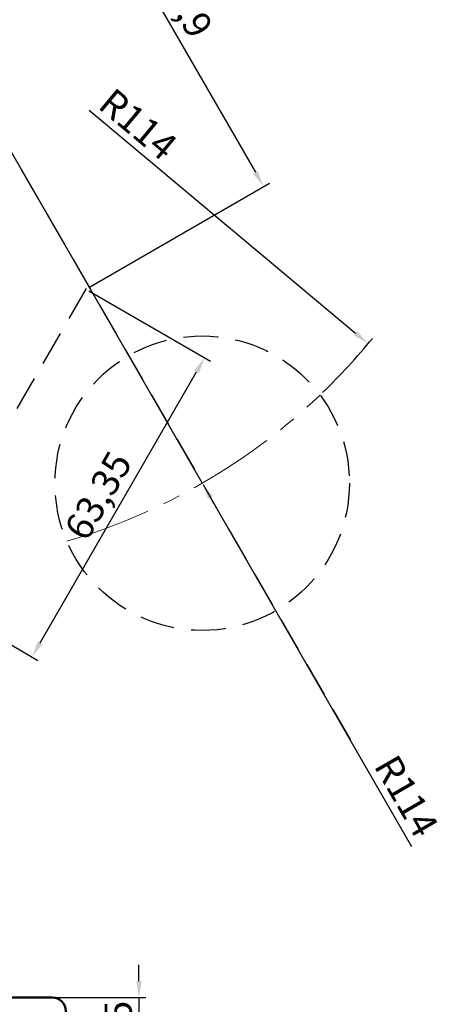
# Model space of a CAD drawing. Units: millimetres. Extents: x 98 to 674, y 38 to 476.
# Tile 5 of 7: x 315 to 392, y 131 to 312. Entities that reach past the tile are written whole.
import ezdxf

# ---------------------------------------------------------------- set-up
doc = ezdxf.new("R2010")
doc.units = ezdxf.units.MM
doc.header["$LTSCALE"] = 0.5
doc.linetypes.add('CENTER', pattern=[50.8, 31.75, -6.35, 6.35, -6.35])
doc.linetypes.add('DASHED', pattern=[19.05, 12.7, -6.35])
for name, color, linetype, lineweight in [('M-CNTR', 1, 'CENTER', 18), ('M-DIMS', 2, 'Continuous', 25), ('M-OUTL', 7, 'Continuous', 50), ('M-PHAN', 6, 'DASHED', 25)]:
    doc.layers.add(name, color=color, linetype=linetype, lineweight=lineweight)
doc.styles.get("Standard").update_dxf_attribs({"font": 'arial.ttf'})
doc.dimstyles.new('ISO-25', dxfattribs={"dimtxt": 5, "dimasz": 3, "dimexe": 1.25, "dimexo": 0.625, "dimtad": 1, "dimtxsty": 'Standard', "dimcen": 2.5, "dimadec": 0, "dimazin": 0, "dimtfac": 1, "dimtmove": 0, "dimatfit": 3, "dimfxl": 1, "dimarcsym": 0})

# ---------------------------------------------------------------- blocks, each defined once
blk = doc.blocks.new('*D20')
at = {"layer": 'Defpoints', "color": 0, "ltscale": 0.5, "transparency": 16777216}
for p in [(290.59, 325.69), (359.62, 281.36), (327.04, 262.55)]:
    blk.add_point(p, dxfattribs=at)
at = {"layer": 'M-DIMS', "color": 0, "lineweight": -2, "ltscale": 0.5, "transparency": 16777216}
for p, q in [((291.13, 326), (324.25, 345.12)), ((324.67, 341.9), (358.12, 283.96)), ((327.58, 262.86), (360.7, 281.99))]:
    blk.add_line(p, q, dxfattribs=at)
at = {"layer": 'M-DIMS', "color": 0, "ltscale": 0.5, "transparency": 16777216}
for points in [[(325.1, 342.15), (324.24, 341.65), (323.17, 344.5)], [(358.56, 284.21), (357.69, 283.71), (359.62, 281.36)]]:
    blk.add_solid(points, dxfattribs=at)
at = {"layer": 'M-DIMS', "color": 0, "ltscale": 0.5, "transparency": 16777216, "insert": (344.54, 314.74), "char_height": 5, "attachment_point": 5, "rotation": 300}
blk.add_mtext('72,9', dxfattribs=at)
blk = doc.blocks.new('*D21')
at = {"layer": 'Defpoints', "color": 0, "ltscale": 0.5, "transparency": 16777216}
for p in [(327.04, 262.55), (348.82, 249.98), (295.37, 207.69)]:
    blk.add_point(p, dxfattribs=at)
at = {"layer": 'M-DIMS', "color": 0, "lineweight": -2, "ltscale": 0.5, "transparency": 16777216}
for p, q in [((327.58, 262.24), (349.9, 249.35)), ((318.64, 197.71), (347.32, 247.38)), ((295.91, 207.37), (318.22, 194.49))]:
    blk.add_line(p, q, dxfattribs=at)
at = {"layer": 'M-DIMS', "color": 0, "ltscale": 0.5, "transparency": 16777216}
for points in [[(346.89, 247.63), (347.75, 247.13), (348.82, 249.98)], [(318.21, 197.96), (319.08, 197.46), (317.14, 195.11)]]:
    blk.add_solid(points, dxfattribs=at)
at = {"layer": 'M-DIMS', "color": 0, "ltscale": 0.5, "transparency": 16777216, "insert": (329.84, 224.36), "char_height": 5, "attachment_point": 5, "rotation": 60}
blk.add_mtext('63,35', dxfattribs=at)
blk = doc.blocks.new('*D22')
at = {"layer": 'Defpoints', "color": 0, "ltscale": 0.5, "transparency": 16777216}
for p in [(291.37, 325.69), (378.81, 252.55)]:
    blk.add_point(p, dxfattribs=at)
at = {"layer": 'M-DIMS', "color": 0, "lineweight": -2, "ltscale": 0.5, "transparency": 16777216}
blk.add_line((327.65, 295.34), (376.51, 254.47), dxfattribs=at)
blk.add_arc((291.37, 325.69), 114, 313.9161, 320.7202, dxfattribs=at)
at = {"layer": 'M-DIMS', "color": 0, "ltscale": 0.5, "transparency": 16777216}
blk.add_solid([(376.83, 254.86), (376.19, 254.09), (378.81, 252.55)], dxfattribs=at)
at = {"layer": 'M-DIMS', "color": 0, "ltscale": 0.5, "transparency": 16777216, "insert": (336.2, 292.27), "char_height": 5, "attachment_point": 5, "rotation": 320.0919}
blk.add_mtext('R114', dxfattribs=at)
blk = doc.blocks.new('*D42')
at = {"layer": 'Defpoints', "color": 0, "ltscale": 0.5, "transparency": 16777216}
for p in [(316.66, 132.69), (316.66, 127.69), (336.77, 127.69)]:
    blk.add_point(p, dxfattribs=at)
at = {"layer": 'M-DIMS', "color": 0, "lineweight": -2, "ltscale": 0.5, "transparency": 16777216}
for p, q in [((336.77, 135.69), (336.77, 138.69)), ((317.29, 132.69), (338.02, 132.69)), ((336.77, 132.69), (336.77, 127.69)), ((317.29, 127.69), (338.02, 127.69)), ((336.77, 124.69), (336.77, 121.69))]:
    blk.add_line(p, q, dxfattribs=at)
at = {"layer": 'M-DIMS', "color": 0, "ltscale": 0.5, "transparency": 16777216}
for points in [[(336.27, 135.69), (337.27, 135.69), (336.77, 132.69)], [(336.27, 124.69), (337.27, 124.69), (336.77, 127.69)]]:
    blk.add_solid(points, dxfattribs=at)
at = {"layer": 'M-DIMS', "color": 0, "ltscale": 0.5, "transparency": 16777216, "insert": (333.6, 130.19), "char_height": 5, "attachment_point": 5, "rotation": 90}
blk.add_mtext('5', dxfattribs=at)
blk = doc.blocks.new('*D72')
at = {"layer": 'Defpoints', "color": 0, "ltscale": 0.5, "transparency": 16777216}
for p in [(149.37, 196.69), (323.37, 130.19), (323.37, 42.76)]:
    blk.add_point(p, dxfattribs=at)
at = {"layer": 'M-DIMS', "color": 0, "lineweight": -2, "ltscale": 0.5, "transparency": 16777216}
for p, q in [((149.37, 196.06), (149.37, 41.51)), ((323.37, 129.56), (323.37, 41.51)), ((152.37, 42.76), (320.37, 42.76))]:
    blk.add_line(p, q, dxfattribs=at)
at = {"layer": 'M-DIMS', "color": 0, "ltscale": 0.5, "transparency": 16777216}
for points in [[(152.37, 43.26), (152.37, 42.26), (149.37, 42.76)], [(320.37, 43.26), (320.37, 42.26), (323.37, 42.76)]]:
    blk.add_solid(points, dxfattribs=at)
at = {"layer": 'M-DIMS', "color": 0, "ltscale": 0.5, "transparency": 16777216, "insert": (236.37, 45.9), "char_height": 5, "attachment_point": 5}
blk.add_mtext('174', dxfattribs=at)
blk = doc.blocks.new('*D78')
at = {"layer": 'Defpoints', "color": 0, "ltscale": 0.5, "transparency": 16777216}
for p in [(291.37, 325.69), (348.37, 226.96)]:
    blk.add_point(p, dxfattribs=at)
at = {"layer": 'M-DIMS', "color": 0, "lineweight": -2, "ltscale": 0.5, "transparency": 16777216}
for p, q in [((291.37, 325.69), (348.37, 226.96)), ((386.83, 160.33), (349.87, 224.36))]:
    blk.add_line(p, q, dxfattribs=at)
at = {"layer": 'M-DIMS', "color": 0, "ltscale": 0.5, "transparency": 16777216}
blk.add_solid([(350.3, 224.61), (349.43, 224.11), (348.37, 226.96)], dxfattribs=at)
at = {"layer": 'M-DIMS', "color": 0, "ltscale": 0.5, "transparency": 16777216, "insert": (385.28, 169.29), "char_height": 5, "attachment_point": 5, "rotation": 300.0001}
blk.add_mtext('R114', dxfattribs=at)

msp = doc.modelspace()

# ---------------------------------------------------------------- linework, layer by layer
at = {"layer": 'M-CNTR'}
msp.add_arc((291.365, 325.6855), 114, 286.398028, 313.601972, dxfattribs=at)
at = {"layer": 'M-OUTL'}
msp.add_lwpolyline([(320.865, 132.6855), (233.865, 132.6855, 1), (233.865, 127.6855), (320.865, 127.6855, 1)], format="xyb", close=True, dxfattribs=at)
at = {"layer": 'M-PHAN'}
for p, q in [((291.365, 325.6855), (375.7053, 179.6039)), ((295.365, 207.6855), (327.4287, 263.2214))]:
    msp.add_line(p, q, dxfattribs=at)
msp.add_circle((348.365, 226.9586), 27, dxfattribs=at)

# ---------------------------------------------------------------- dimensions: what is measured, and where the dimension line sits
at = {"layer": 'M-DIMS', "ltscale": 0.5}
for p1, distance, picture, middle in [((290.5915, 325.6855), 37.6203, '*D20', (344.5403, 314.7435)), ((295.365, 207.6855), -25.146, '*D21', (329.8371, 224.3604))]:
    dim = msp.add_aligned_dim(p1=p1, p2=(327.0419, 262.5515), distance=distance, dimstyle='ISO-25', override={"dimclrd": 0, "dimclre": 0, "dimclrt": 0}, dxfattribs=at)
    dim.commit()
    dim.dimension.update_dxf_attribs({"geometry": picture, "text_midpoint": middle})
for mpoint, override, picture, middle in [((378.8115, 252.5479), {"dimclrd": 0, "dimclre": 0, "dimclrt": 0}, '*D22', (334.1894, 289.8685)), ((348.3652, 226.9587), {"dimdec": 0, "dimlfac": 1, "dimrnd": 0, "dimzin": 0, "dimdsep": 46, "dimlunit": 2}, '*D78', (382.5653, 167.7226))]:
    dim = msp.add_radius_dim(center=(291.365, 325.6855), mpoint=mpoint, dimstyle='ISO-25', override=override, dxfattribs=at)
    dim.commit()
    dim.dimension.update_dxf_attribs({"geometry": picture, "text_midpoint": middle, "dimtype": 164})
dim = msp.add_linear_dim(base=(323.365, 42.7639), p1=(149.365, 196.6855), p2=(323.365, 130.1855), dimstyle='ISO-25', override={"dimdec": 0, "dimlfac": 1, "dimrnd": 0, "dimzin": 0, "dimdsep": 46, "dimlunit": 2}, dxfattribs=at)
dim.commit()
dim.dimension.update_dxf_attribs({"geometry": '*D72', "text_midpoint": (236.365, 45.8992)})
dim = msp.add_linear_dim(base=(336.7704, 127.6855), p1=(316.6618, 132.6855), p2=(316.6618, 127.6855), angle=90, dimstyle='ISO-25', override={"dimclrd": 0, "dimclre": 0, "dimclrt": 0}, dxfattribs=at)
dim.commit()
dim.dimension.update_dxf_attribs({"geometry": '*D42', "text_midpoint": (333.6027, 130.1855)})

doc.saveas('drawing.dxf')
